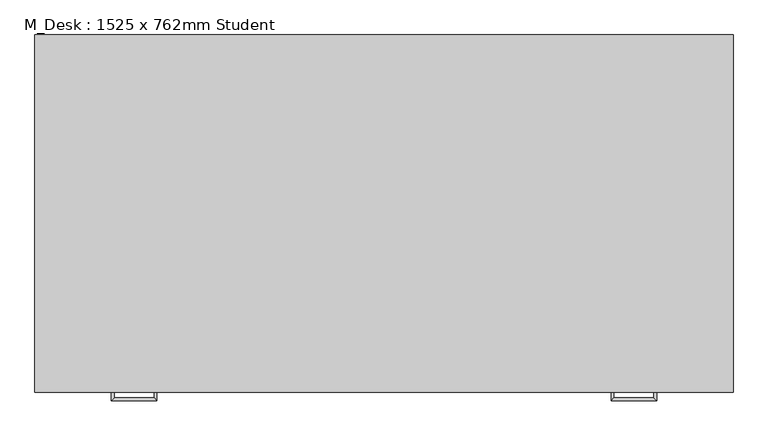
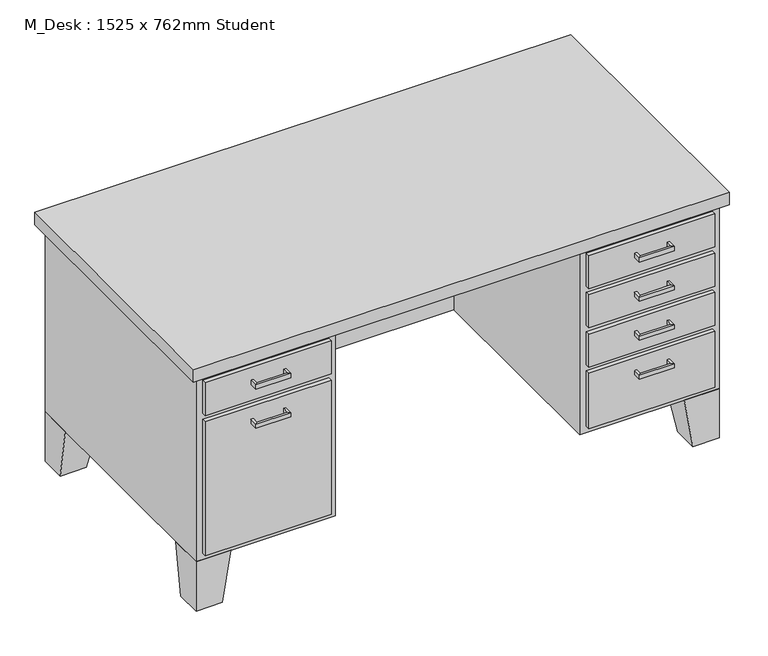
"""IFC4 building model written with IfcOpenShell, lengths in millimetres: furniture geometry, M_Desk : 1525 x 762mm Student."""

from ifc_helpers import new_model, si_unit, frame, origin, place, context, project, spatial, polyline, outline, extrude, faceted_brep, source, transform, mapped, element, save


def m_desk_1525_x_762mm_student_8f660baf(model_context):
    return source(origin(), model_context, "Body", "SolidModel", [
        extrude(outline(polyline([(18.55, 0.0), (386.85, 0.0), (386.85, -12.7), (18.55, -12.7), (18.55, 0.0)])), frame((0.0, 0.0, 603.25), z_axis=(0.0, 0.0, 1.0), x_axis=(1.0, 0.0, 0.0)), (0.0, 0.0, 1.0), 101.6),
        extrude(outline(polyline([(18.55, 0.0), (386.85, 0.0), (386.85, -12.7), (18.55, -12.7), (18.55, 0.0)])), frame((0.0, 0.0, 171.05), z_axis=(0.0, 0.0, 1.0), x_axis=(1.0, 0.0, 0.0)), (0.0, 0.0, 1.0), 413.15),
        extrude(outline(polyline([(1137.15, 0.0), (1505.45, 0.0), (1505.45, -12.7), (1137.15, -12.7), (1137.15, 0.0)])), frame((0.0, 0.0, 602.85), z_axis=(0.0, 0.0, 1.0), x_axis=(1.0, 0.0, 0.0)), (0.0, 0.0, 1.0), 102.0),
        extrude(outline(polyline([(1137.15, 0.0), (1505.45, 0.0), (1505.45, -12.7), (1137.15, -12.7), (1137.15, 0.0)])), frame((0.0, 0.0, 171.05), z_axis=(0.0, 0.0, 1.0), x_axis=(1.0, 0.0, 0.0)), (0.0, 0.0, 1.0), 171.45),
        extrude(outline(polyline([(1137.15, 0.0), (1505.45, 0.0), (1505.45, -12.7), (1137.15, -12.7), (1137.15, 0.0)])), frame((0.0, 0.0, 482.2), z_axis=(0.0, 0.0, 1.0), x_axis=(1.0, 0.0, 0.0)), (0.0, 0.0, 1.0), 101.6),
        extrude(outline(polyline([(1137.15, 0.0), (1505.45, 0.0), (1505.45, -12.7), (1137.15, -12.7), (1137.15, 0.0)])), frame((0.0, 0.0, 361.55), z_axis=(0.0, 0.0, 1.0), x_axis=(1.0, 0.0, 0.0)), (0.0, 0.0, 1.0), 101.6),
        faceted_brep([(101.1, 0.0, 152.0), (101.1, 101.6, 152.0), (-0.5, 101.6, 152.0), (-0.5, 0.0, 152.0), (75.7, 0.0, 0.0), (-0.5, 0.0, 0.0), (-0.5, 76.2, 0.0), (75.7, 76.2, 0.0)], [[[0, 1, 2, 3]], [[4, 5, 6, 7]], [[4, 7, 1, 0]], [[7, 6, 2, 1]], [[6, 5, 3, 2]], [[5, 4, 0, 3]]]),
        faceted_brep([(101.1, 762.0, 152.0), (-0.5, 762.0, 152.0), (-0.5, 660.4, 152.0), (101.1, 660.4, 152.0), (75.7, 762.0, 0.0), (75.7, 685.8, 0.0), (-0.5, 685.8, 0.0), (-0.5, 762.0, 0.0)], [[[0, 1, 2, 3]], [[4, 5, 6, 7]], [[4, 7, 1, 0]], [[7, 6, 2, 1]], [[6, 5, 3, 2]], [[5, 4, 0, 3]]]),
        faceted_brep([(1422.9, 762.0, 152.0), (1422.9, 660.4, 152.0), (1524.5, 660.4, 152.0), (1524.5, 762.0, 152.0), (1448.3, 762.0, 0.0), (1524.5, 762.0, 0.0), (1524.5, 685.8, 0.0), (1448.3, 685.8, 0.0)], [[[0, 1, 2, 3]], [[4, 5, 6, 7]], [[4, 7, 1, 0]], [[7, 6, 2, 1]], [[6, 5, 3, 2]], [[5, 4, 0, 3]]]),
        faceted_brep([(1422.9, 0.0, 152.0), (1524.5, 0.0, 152.0), (1524.5, 101.6, 152.0), (1422.9, 101.6, 152.0), (1448.3, 0.0, 0.0), (1448.3, 76.2, 0.0), (1524.5, 76.2, 0.0), (1524.5, 0.0, 0.0)], [[[0, 1, 2, 3]], [[4, 5, 6, 7]], [[4, 7, 1, 0]], [[7, 6, 2, 1]], [[6, 5, 3, 2]], [[5, 4, 0, 3]]]),
        extrude(outline(polyline([(-19.55, -19.05), (-19.55, 781.05), (1543.55, 781.05), (1543.55, -19.05), (-19.55, -19.05)])), frame((0.0, 0.0, 723.9), z_axis=(0.0, 0.0, 1.0), x_axis=(1.0, 0.0, 0.0)), (0.0, 0.0, 1.0), 38.1),
        extrude(outline(polyline([(1118.1, 0.0), (1118.1, 635.0), (405.9, 635.0), (405.9, 0.0), (-0.5, 0.0), (-0.5, 762.0), (1524.5, 762.0), (1524.5, 0.0), (1118.1, 0.0)])), frame((0.0, 0.0, 152.0), z_axis=(0.0, 0.0, 1.0), x_axis=(1.0, 0.0, 0.0)), (0.0, 0.0, 1.0), 571.9),
        faceted_brep([(158.25, -12.7, 546.1), (158.25, -12.7, 533.4), (151.9, -12.7, 533.4), (151.9, -12.7, 546.1), (158.25, -31.75, 546.1), (158.25, -31.75, 533.4), (151.9, -38.1, 533.4), (151.9, -38.1, 546.1), (247.15, -31.75, 546.1), (247.15, -31.75, 533.4), (253.5, -38.1, 533.4), (253.5, -38.1, 546.1), (247.15, -12.7, 546.1), (253.5, -12.7, 546.1), (253.5, -12.7, 533.4), (247.15, -12.7, 533.4)], [[[0, 1, 2, 3]], [[1, 0, 4, 5]], [[2, 1, 5, 6]], [[3, 2, 6, 7]], [[0, 3, 7, 4]], [[5, 4, 8, 9]], [[6, 5, 9, 10]], [[7, 6, 10, 11]], [[4, 7, 11, 8]], [[12, 13, 14, 15]], [[9, 8, 12, 15]], [[10, 9, 15, 14]], [[11, 10, 14, 13]], [[8, 11, 13, 12]]]),
        faceted_brep([(158.25, -12.7, 666.75), (158.25, -12.7, 654.05), (151.9, -12.7, 654.05), (151.9, -12.7, 666.75), (158.25, -31.75, 666.75), (158.25, -31.75, 654.05), (151.9, -38.1, 654.05), (151.9, -38.1, 666.75), (247.15, -31.75, 666.75), (247.15, -31.75, 654.05), (253.5, -38.1, 654.05), (253.5, -38.1, 666.75), (247.15, -12.7, 666.75), (253.5, -12.7, 666.75), (253.5, -12.7, 654.05), (247.15, -12.7, 654.05)], [[[0, 1, 2, 3]], [[1, 0, 4, 5]], [[2, 1, 5, 6]], [[3, 2, 6, 7]], [[0, 3, 7, 4]], [[5, 4, 8, 9]], [[6, 5, 9, 10]], [[7, 6, 10, 11]], [[4, 7, 11, 8]], [[12, 13, 14, 15]], [[9, 8, 12, 15]], [[10, 9, 15, 14]], [[11, 10, 14, 13]], [[8, 11, 13, 12]]]),
        faceted_brep([(1365.75, -12.7, 304.8), (1372.1, -12.7, 304.8), (1372.1, -12.7, 292.1), (1365.75, -12.7, 292.1), (1365.75, -31.75, 304.8), (1372.1, -38.1, 304.8), (1372.1, -38.1, 292.1), (1365.75, -31.75, 292.1), (1276.85, -31.75, 304.8), (1270.5, -38.1, 304.8), (1270.5, -38.1, 292.1), (1276.85, -31.75, 292.1), (1276.85, -12.7, 304.8), (1276.85, -12.7, 292.1), (1270.5, -12.7, 292.1), (1270.5, -12.7, 304.8)], [[[0, 1, 2, 3]], [[1, 0, 4, 5]], [[2, 1, 5, 6]], [[3, 2, 6, 7]], [[0, 3, 7, 4]], [[5, 4, 8, 9]], [[6, 5, 9, 10]], [[7, 6, 10, 11]], [[4, 7, 11, 8]], [[12, 13, 14, 15]], [[9, 8, 12, 15]], [[10, 9, 15, 14]], [[11, 10, 14, 13]], [[8, 11, 13, 12]]]),
        faceted_brep([(1365.75, -12.7, 425.45), (1372.1, -12.7, 425.45), (1372.1, -12.7, 412.75), (1365.75, -12.7, 412.75), (1365.75, -31.75, 425.45), (1372.1, -38.1, 425.45), (1372.1, -38.1, 412.75), (1365.75, -31.75, 412.75), (1276.85, -31.75, 425.45), (1270.5, -38.1, 425.45), (1270.5, -38.1, 412.75), (1276.85, -31.75, 412.75), (1276.85, -12.7, 425.45), (1276.85, -12.7, 412.75), (1270.5, -12.7, 412.75), (1270.5, -12.7, 425.45)], [[[0, 1, 2, 3]], [[1, 0, 4, 5]], [[2, 1, 5, 6]], [[3, 2, 6, 7]], [[0, 3, 7, 4]], [[5, 4, 8, 9]], [[6, 5, 9, 10]], [[7, 6, 10, 11]], [[4, 7, 11, 8]], [[12, 13, 14, 15]], [[9, 8, 12, 15]], [[10, 9, 15, 14]], [[11, 10, 14, 13]], [[8, 11, 13, 12]]]),
        faceted_brep([(1365.75, -12.7, 546.1), (1372.1, -12.7, 546.1), (1372.1, -12.7, 533.4), (1365.75, -12.7, 533.4), (1365.75, -31.75, 546.1), (1372.1, -38.1, 546.1), (1372.1, -38.1, 533.4), (1365.75, -31.75, 533.4), (1276.85, -31.75, 546.1), (1270.5, -38.1, 546.1), (1270.5, -38.1, 533.4), (1276.85, -31.75, 533.4), (1276.85, -12.7, 546.1), (1276.85, -12.7, 533.4), (1270.5, -12.7, 533.4), (1270.5, -12.7, 546.1)], [[[0, 1, 2, 3]], [[1, 0, 4, 5]], [[2, 1, 5, 6]], [[3, 2, 6, 7]], [[0, 3, 7, 4]], [[5, 4, 8, 9]], [[6, 5, 9, 10]], [[7, 6, 10, 11]], [[4, 7, 11, 8]], [[12, 13, 14, 15]], [[9, 8, 12, 15]], [[10, 9, 15, 14]], [[11, 10, 14, 13]], [[8, 11, 13, 12]]]),
        faceted_brep([(1365.75, -12.7, 666.75), (1372.1, -12.7, 666.75), (1372.1, -12.7, 654.05), (1365.75, -12.7, 654.05), (1365.75, -31.75, 666.75), (1372.1, -38.1, 666.75), (1372.1, -38.1, 654.05), (1365.75, -31.75, 654.05), (1276.85, -31.75, 666.75), (1270.5, -38.1, 666.75), (1270.5, -38.1, 654.05), (1276.85, -31.75, 654.05), (1276.85, -12.7, 666.75), (1276.85, -12.7, 654.05), (1270.5, -12.7, 654.05), (1270.5, -12.7, 666.75)], [[[0, 1, 2, 3]], [[1, 0, 4, 5]], [[2, 1, 5, 6]], [[3, 2, 6, 7]], [[0, 3, 7, 4]], [[5, 4, 8, 9]], [[6, 5, 9, 10]], [[7, 6, 10, 11]], [[4, 7, 11, 8]], [[12, 13, 14, 15]], [[9, 8, 12, 15]], [[10, 9, 15, 14]], [[11, 10, 14, 13]], [[8, 11, 13, 12]]]),
    ])


if __name__ == "__main__":
    model = new_model("IFC4")
    model_context = context("Model", 3, world=origin())
    ifc_project = project(units=[si_unit("LENGTHUNIT", "METRE", prefix="MILLI")], contexts=[model_context])
    site = spatial("IfcSite", under=ifc_project)
    building = spatial("IfcBuilding", under=site)
    placement = place(None, origin())
    m_desk_1525_x_762mm_student_shape = m_desk_1525_x_762mm_student_8f660baf(model_context)
    element("IfcFurniture", 1, ObjectType="M_Desk : 1525 x 762mm Student", at=placement, inside=building, context=model_context, shape_type="MappedRepresentation", body=[
        mapped(m_desk_1525_x_762mm_student_shape, transform((0.0, 0.0, 0.0), x_axis=(1.0, 0.0, 0.0), y_axis=(0.0, 1.0, 0.0), z_axis=(0.0, 0.0, 1.0))),
    ])
    save(model, "model.ifc")

# Revit data of these elements
# Type "M_Desk : 1525 x 762mm Student"
#   Depth = 762 mm
#   Height = 762 mm
#   Leg Height = 152 mm
#   Width = 1525 mm
#   Body Material = Laminate, Ivory, Matte
#   Handle/Leg Material = Steel, Chrome Plated
#   Top Material = Cherry
#   Default Elevation = 0
#   Assembly Code = ""
# Element 1 (IfcFurniture, "M_Desk : 1525 x 762mm Student")
#   Materials on its faces: "Steel, Chrome Plated", "Laminate, Ivory, Matte", "Cherry"
# Materials
#   "Laminate, Ivory, Matte": class "Plastic", colour RGB 247 247 239, transparency 0, Description = "Plastic Laminate - Ivory, Matte", Cost = 0
#   "Steel, Chrome Plated": class "Metal", colour RGB 17 17 17, transparency 0, Description = "Chromiuim plated steel", Cost = 0
#   "Cherry": class "Wood", colour RGB 226 177 128, transparency 0, Description = "Prunus Serotina", Cost = 0
